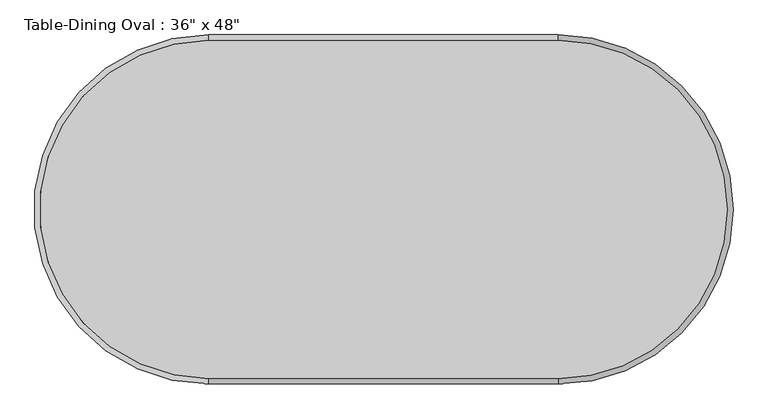
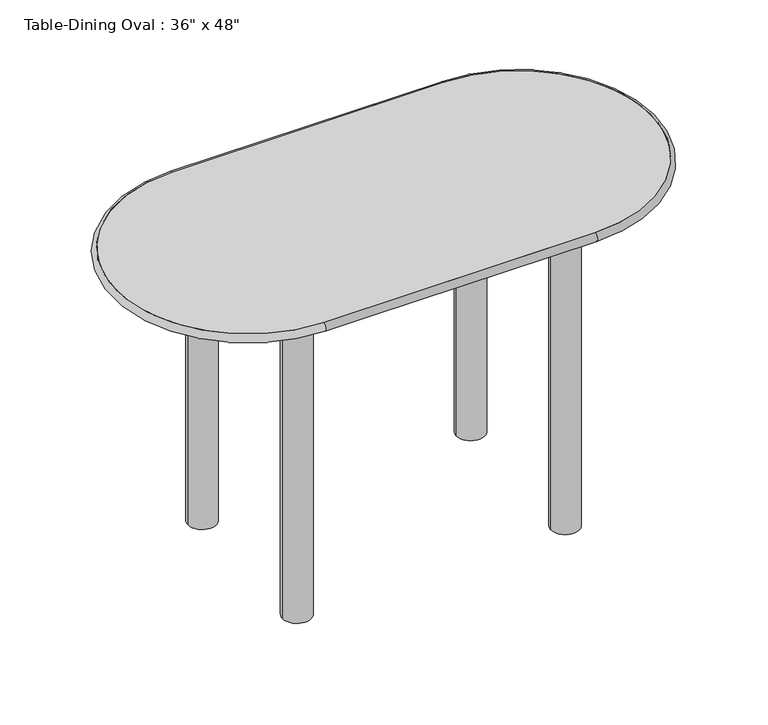
"""IFC4 building model written with IfcOpenShell, lengths in millimetres: furniture geometry."""

from ifc_helpers import new_model, si_unit, point, frame, frame_2d, origin, origin_with_axes, place, context, project, spatial, polyline, circle_curve, ellipse_curve, trimmed, segment, composite_curve, outline, extrude, source, transform, mapped, element, save
from ifc_brep_helpers import plane_surface, cylinder_surface, revolved_surface, advanced_brep


def furniture_6551fbda(model_context):
    return source(origin(), model_context, "Body", "SolidModel", [
        advanced_brep(
        [(-706.6196721, -653.3733607, 762.0), (-706.6196721, -653.3733607, 742.95), (-97.0196721, -653.3733607, 742.95), (-97.0196721, -653.3733607, 762.0), (-97.0196721, -62.8233607, 762.0), (-97.0196721, -62.8233607, 742.95), (-706.6196721, -62.8233607, 742.95), (-706.6196721, -62.8233607, 762.0)],
        [
            (0, 1, circle_curve(frame((-706.6196721, -653.3733607, 752.475), z_axis=(1.0, 0.0, 0.0), x_axis=(0.0, 1.0, 0.0)), 9.525)),
            (1, 2),
            (2, 3, circle_curve(frame((-97.0196721, -653.3733607, 752.475), z_axis=(-1.0, 0.0, 0.0), x_axis=(0.0, 1.0, 0.0)), 9.525)),
            (3, 0),
            (1, 0),
            (3, 2),
            (4, 3, circle_curve(frame((-97.0196721, -358.0983607, 762.0), z_axis=(0.0, 0.0, -1.0), x_axis=(0.0, -1.0, 0.0)), 295.275)),
            (2, 5, circle_curve(frame((-97.0196721, -358.0983607, 742.95), z_axis=(0.0, 0.0, 1.0), x_axis=(0.0, -1.0, 0.0)), 295.275)),
            (5, 4, circle_curve(frame((-97.0196721, -62.8233607, 752.475), z_axis=(1.0, 0.0, 0.0), x_axis=(0.0, -1.0, 0.0)), 9.525)),
            (4, 5),
            (5, 6),
            (6, 7, circle_curve(frame((-706.6196721, -62.8233607, 752.475), z_axis=(1.0, 0.0, 0.0), x_axis=(0.0, -1.0, 0.0)), 9.525)),
            (7, 4),
            (7, 6),
            (0, 7, circle_curve(frame((-706.6196721, -358.0983607, 762.0), z_axis=(0.0, 0.0, -1.0), x_axis=(0.0, 1.0, 0.0)), 295.275)),
            (6, 1, circle_curve(frame((-706.6196721, -358.0983607, 742.95), z_axis=(0.0, 0.0, 1.0), x_axis=(0.0, 1.0, 0.0)), 295.275)),
        ],
        [
            cylinder_surface(frame((-706.6196721, -653.3733607, 752.475), z_axis=(-1.0, 0.0, 0.0), x_axis=(0.0, 1.0, 0.0)), 9.525),
            plane_surface(frame((-706.6196721, -653.3733607, 762.0), z_axis=(0.0, 1.0, 0.0), x_axis=(1.0, 0.0, 0.0))),
            revolved_surface(trimmed(ellipse_curve(frame((-97.0196721, -653.3733607, 752.475), z_axis=(-1.0, 0.0, 0.0), x_axis=(0.0, 1.0, 0.0)), 9.525, 9.525), [point((-97.0196721, -653.3733607, 742.95))], [point((-97.0196721, -653.3733607, 762.0))], True, "CARTESIAN"), (-97.0196721, -358.0983607, 0.0), (0.0, 0.0, 1.0)),
            revolved_surface(polyline([(-97.0196721, -653.3733606999999, 762.0), (-97.0196721, -653.3733606999999, 742.95)]), (-97.0196721, -358.0983607, 0.0), (0.0, 0.0, 1.0)),
            cylinder_surface(frame((-97.0196721, -62.8233607, 752.475), z_axis=(1.0, 0.0, 0.0), x_axis=(0.0, -1.0, 0.0)), 9.525),
            plane_surface(frame((-97.0196721, -62.8233607, 762.0), z_axis=(0.0, -1.0, 0.0), x_axis=(-1.0, 0.0, 0.0))),
            revolved_surface(trimmed(ellipse_curve(frame((-706.6196721, -62.8233607, 752.475), z_axis=(1.0, 0.0, 0.0), x_axis=(0.0, -1.0, 0.0)), 9.525, 9.525), [point((-706.6196721, -62.8233607, 742.95))], [point((-706.6196721, -62.8233607, 762.0))], True, "CARTESIAN"), (-706.6196721, -358.0983607, 0.0), (0.0, 0.0, 1.0)),
            revolved_surface(polyline([(-706.6196721, -62.82336070000002, 762.0), (-706.6196721, -62.82336070000002, 742.95)]), (-706.6196721, -358.0983607, 0.0), (0.0, 0.0, 1.0)),
        ],
        [
            (0, [[1, 2, 3, 4]]),
            (1, [[5, -4, 6, -2]]),
            (2, [[7, -3, 8, 9]]),
            (3, [[-8, -6, -7, 10]]),
            (4, [[-9, 11, 12, 13]]),
            (5, [[-10, -13, 14, -11]]),
            (6, [[15, -12, 16, -1]]),
            (7, [[-16, -14, -15, -5]]),
        ],
    ),
        extrude(outline(composite_curve([segment(trimmed(circle_curve(frame_2d((-703.4446721, -173.9483607)), 31.75), [point((-735.1946721, -173.9483607))], [point((-671.6946721, -173.9483607))], False, "CARTESIAN"), True, "CONTINUOUS"), segment(trimmed(circle_curve(frame_2d((-703.4446721, -173.9483607)), 31.75), [point((-671.6946721, -173.9483607))], [point((-735.1946721, -173.9483607))], False, "CARTESIAN"), True, "CONTINUOUS")], self_intersect=False)), origin_with_axes(), (0.0, 0.0, 1.0), 742.95),
        extrude(outline(composite_curve([segment(trimmed(circle_curve(frame_2d((-703.4446721, -542.2483607)), 31.75), [point((-735.1946721, -542.2483607))], [point((-671.6946721, -542.2483607))], False, "CARTESIAN"), True, "CONTINUOUS"), segment(trimmed(circle_curve(frame_2d((-703.4446721, -542.2483607)), 31.75), [point((-671.6946721, -542.2483607))], [point((-735.1946721, -542.2483607))], False, "CARTESIAN"), True, "CONTINUOUS")], self_intersect=False)), origin_with_axes(), (0.0, 0.0, 1.0), 742.95),
        extrude(outline(composite_curve([segment(trimmed(circle_curve(frame_2d((-100.1946721, -173.9483607)), 31.75), [point((-131.9446721, -173.9483607))], [point((-68.4446721, -173.9483607))], False, "CARTESIAN"), True, "CONTINUOUS"), segment(trimmed(circle_curve(frame_2d((-100.1946721, -173.9483607)), 31.75), [point((-68.4446721, -173.9483607))], [point((-131.9446721, -173.9483607))], False, "CARTESIAN"), True, "CONTINUOUS")], self_intersect=False)), origin_with_axes(), (0.0, 0.0, 1.0), 742.95),
        extrude(outline(composite_curve([segment(trimmed(circle_curve(frame_2d((-100.1946721, -542.2483607)), 31.75), [point((-131.9446721, -542.2483607))], [point((-68.4446721, -542.2483607))], False, "CARTESIAN"), True, "CONTINUOUS"), segment(trimmed(circle_curve(frame_2d((-100.1946721, -542.2483607)), 31.75), [point((-68.4446721, -542.2483607))], [point((-131.9446721, -542.2483607))], False, "CARTESIAN"), True, "CONTINUOUS")], self_intersect=False)), origin_with_axes(), (0.0, 0.0, 1.0), 742.95),
        extrude(outline(polyline([(-81.1446721, -154.8983607), (-81.1446721, -561.2983607), (-722.4946721, -561.2983607), (-722.4946721, -154.8983607), (-81.1446721, -154.8983607)]), holes=[polyline([(-100.1946721, -173.9483607), (-703.4446721, -173.9483607), (-703.4446721, -542.2483607), (-100.1946721, -542.2483607), (-100.1946721, -173.9483607)])]), frame((0.0, 0.0, 692.15), z_axis=(0.0, 0.0, 1.0), x_axis=(1.0, 0.0, 0.0)), (0.0, 0.0, 1.0), 50.8),
        extrude(outline(composite_curve([segment(polyline([(-706.6196721, -62.8233607), (-97.0196721, -62.8233607)]), True, "CONTINUOUS"), segment(trimmed(circle_curve(frame_2d((-97.0196721, -358.0983607)), 295.275), [point((-97.0196721, -62.8233607))], [point((198.2553279, -358.0983607))], False, "CARTESIAN"), True, "CONTINUOUS"), segment(trimmed(circle_curve(frame_2d((-97.0196721, -358.0983607)), 295.275), [point((198.2553279, -358.0983607))], [point((-97.0196721, -653.3733607))], False, "CARTESIAN"), True, "CONTINUOUS"), segment(polyline([(-97.0196721, -653.3733607), (-706.6196721, -653.3733607)]), True, "CONTINUOUS"), segment(trimmed(circle_curve(frame_2d((-706.6196721, -358.0983607)), 295.275), [point((-706.6196721, -653.3733607))], [point((-1001.8946721, -358.0983607))], False, "CARTESIAN"), True, "CONTINUOUS"), segment(trimmed(circle_curve(frame_2d((-706.6196721, -358.0983607)), 295.275), [point((-1001.8946721, -358.0983607))], [point((-706.6196721, -62.8233607))], False, "CARTESIAN"), True, "CONTINUOUS")], self_intersect=False)), frame((0.0, 0.0, 742.95), z_axis=(0.0, 0.0, 1.0), x_axis=(1.0, 0.0, 0.0)), (0.0, 0.0, 1.0), 19.05),
    ])


if __name__ == "__main__":
    model = new_model("IFC4")
    model_context = context("Model", 3, world=origin())
    ifc_project = project(units=[si_unit("LENGTHUNIT", "METRE", prefix="MILLI")], contexts=[model_context])
    site = spatial("IfcSite", under=ifc_project)
    building = spatial("IfcBuilding", under=site)
    placement = place(None, origin())
    furniture_shape = furniture_6551fbda(model_context)
    element("IfcFurniture", 1, ObjectType="Table-Dining Oval : 36\" x 48\"", at=placement, inside=building, context=model_context, shape_type="MappedRepresentation", body=[
        mapped(furniture_shape, transform((0.0, 0.0, 0.0), x_axis=(1.0, 0.0, 0.0), y_axis=(0.0, 1.0, 0.0), z_axis=(0.0, 0.0, 1.0))),
    ])
    save(model, "model.ifc")

# Revit data of these elements
# Type "Table-Dining Oval : 36\" x 48\""
#   Assembly Code = "E2020200"
#   Length = 4' - 0"
#   Width = 2' - 0"
#   Base Material = Steel, Chrome Plated
#   Top Material = Glass - Clear, Grey
#   Default Elevation = 0
#   Description = (empty or 0)
# Element 1 (IfcFurniture, "Table-Dining Oval : 36\" x 48\"")
#   Materials on its faces: "Steel, Chrome Plated", "Glass - Clear, Grey"
# Materials
#   "Steel, Chrome Plated": class "Metal", colour RGB 17 17 17, transparency 0, Description = "Chromiuim plated steel", Cost = 0
#   "Glass - Clear, Grey": class "Glass", colour RGB 252 255 255, transparency 0.64
